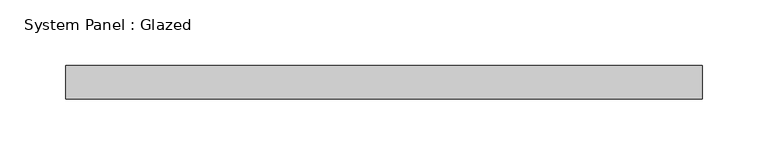
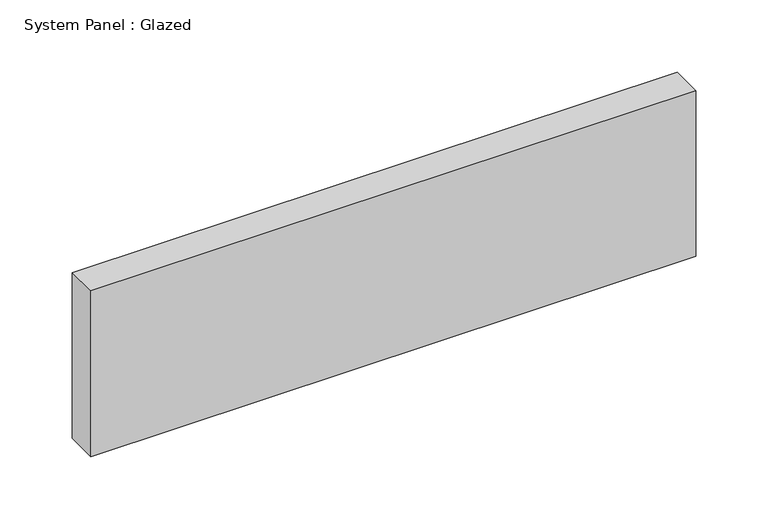
"""IFC4 building model written with IfcOpenShell, lengths in millimetres: plate geometry, System Panel : Glazed."""

from ifc_helpers import new_model, si_unit, origin, origin_with_axes, place, context, project, spatial, polyline, outline, extrude, source, transform, mapped, element, save


def system_panel_glazed_008e37cc(model_context):
    return source(origin(), model_context, "Body", "SweptSolid", [
        extrude(outline(polyline([(241.3, 19.05), (-241.3, 19.05), (-241.3, 44.45), (241.3, 44.45), (241.3, 19.05)])), origin_with_axes(), (0.0, 0.0, 1.0), 139.7),
    ])


if __name__ == "__main__":
    model = new_model("IFC4")
    model_context = context("Model", 3, world=origin())
    ifc_project = project(units=[si_unit("LENGTHUNIT", "METRE", prefix="MILLI")], contexts=[model_context])
    site = spatial("IfcSite", under=ifc_project)
    building = spatial("IfcBuilding", under=site)
    placement = place(None, origin())
    system_panel_glazed_shape = system_panel_glazed_008e37cc(model_context)
    element("IfcPlate", 1, ObjectType="System Panel : Glazed", at=placement, inside=building, context=model_context, shape_type="MappedRepresentation", body=[
        mapped(system_panel_glazed_shape, transform((0.0, 0.0, 0.0), x_axis=(1.0, 0.0, 0.0), y_axis=(0.0, 1.0, 0.0), z_axis=(0.0, 0.0, 1.0))),
    ])
    save(model, "model.ifc")

# Revit data of these elements
# Type "System Panel : Glazed"
#   Construction Type Id = "GSP4R"
#   Analytic Construction = "1/8 in Pilkington single glazing"
#   Visual Light Transmittance = 0.9
#   Solar Heat Gain Coefficient = 0.86
#   Heat Transfer Coefficient (U) = 1.18115 BTU/(h·ft²·°F)
#   Define Thermal Properties by = 1
# Element 1 (IfcPlate, "System Panel : Glazed")
#   Materials on its faces: "Glass"
# Materials
#   "Glass": class "Glass", colour RGB 0 128 192, transparency 0.75, Description = "Soda Lime Glass", Cost = 0
